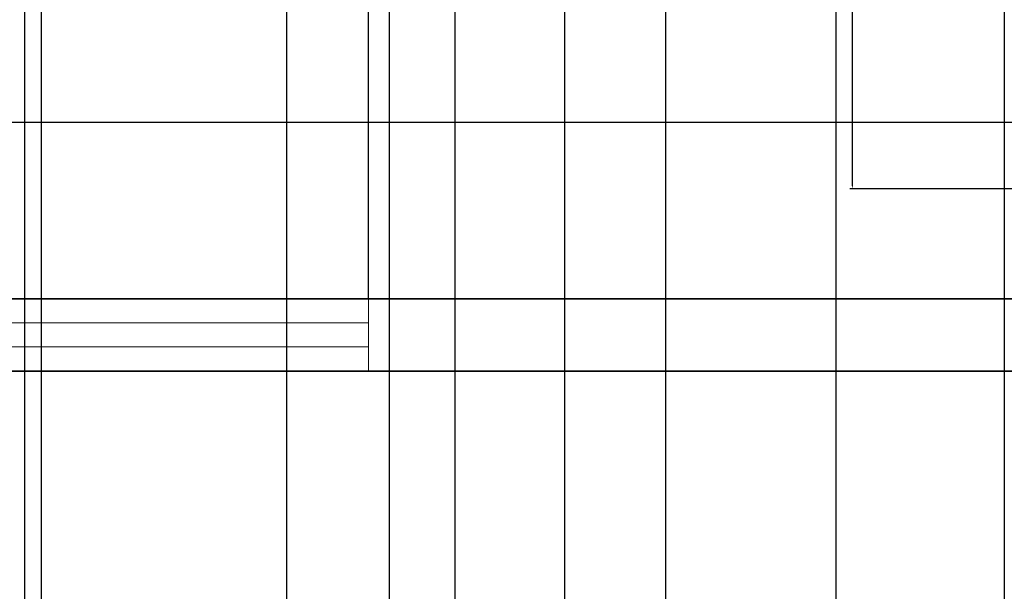
# Model space of a CAD drawing. Units: inches. Extents: x -26 to 385, y 12 to 697.
# Tile 5 of 13: x 223 to 285, y 130 to 165. Entities that reach past the tile are written whole.
import ezdxf

# ---------------------------------------------------------------- set-up
doc = ezdxf.new("R2010")
doc.units = ezdxf.units.IN
doc.header["$MEASUREMENT"] = 0
for name, color, linetype, lineweight in [('A-ANNO-DIMS', 4, 'Continuous', 18), ('A-GLAZ', 5, 'Continuous', 18), ('A-WALL', 40, 'Continuous', 35)]:
    doc.layers.add(name, color=color, linetype=linetype, lineweight=lineweight)
doc.styles.get("Standard").update_dxf_attribs({"font": 'italic8.shx'})
doc.dimstyles.get("Standard").update_dxf_attribs({"dimtxt": 8, "dimasz": 0.18, "dimexe": 0.18, "dimexo": 0.0625, "dimgap": 0.09, "dimtad": 0, "dimtih": 1, "dimtoh": 1, "dimdec": 4, "dimzin": 0, "dimdsep": 46, "dimlunit": 3, "dimtxsty": 'Standard', "dimcen": 0.09, "dimclrd": 2, "dimclre": 3, "dimclrt": 6, "dimadec": 0, "dimazin": 0, "dimtfac": 1, "dimtdec": 4, "dimtofl": 0, "dimtmove": 0, "dimatfit": 3, "dimfxl": 1, "dimtolj": 1, "dimtzin": 0, "dimarcsym": 0})

# ---------------------------------------------------------------- blocks, each defined once
blk = doc.blocks.new('*D11')
at = {"layer": 'A-ANNO-DIMS', "color": 3, "lineweight": -2, "transparency": 16777216}
for p, q in [((285.56, 224.402), (274.992, 224.402)), ((285.56, 154.738), (274.992, 154.738))]:
    blk.add_line(p, q, dxfattribs=at)
at = {"layer": 'A-ANNO-DIMS', "color": 2, "lineweight": -2, "transparency": 16777216}
for p, q in [((275.172, 224.222), (275.172, 195.755)), ((275.172, 154.918), (275.172, 183.384))]:
    blk.add_line(p, q, dxfattribs=at)
at = {"layer": 'A-ANNO-DIMS', "color": 2, "transparency": 16777216}
for points in [[(275.142, 224.222), (275.202, 224.222), (275.172, 224.402)], [(275.142, 154.918), (275.202, 154.918), (275.172, 154.738)]]:
    blk.add_solid(points, dxfattribs=at)
at = {"layer": 'Defpoints', "color": 0, "transparency": 16777216}
for p in [(285.622, 224.402), (275.172, 154.738), (285.622, 154.738)]:
    blk.add_point(p, dxfattribs=at)
at = {"layer": 'A-ANNO-DIMS', "color": 6, "transparency": 16777216, "insert": (275.172, 189.57), "char_height": 8, "attachment_point": 5}
blk.add_mtext('\\A1;SOFA 5\'-9 1/2" TYP.', dxfattribs=at)
blk = doc.blocks.new('*D25')
at = {"layer": 'A-ANNO-DIMS', "color": 3, "lineweight": -2, "transparency": 16777216}
for p, q in [((284.629322, 368.316588), (284.629322, 23.949088)), ((320.629322, 368.316588), (320.629322, 23.949088))]:
    blk.add_line(p, q, dxfattribs=at)
at = {"layer": 'A-ANNO-DIMS', "color": 2, "lineweight": -2, "transparency": 16777216}
for p, q in [((284.449322, 24.129088), (284.269322, 24.129088)), ((320.809322, 24.129088), (320.989322, 24.129088))]:
    blk.add_line(p, q, dxfattribs=at)
at = {"layer": 'A-ANNO-DIMS', "color": 2, "transparency": 16777216}
for points in [[(284.449322, 24.159088), (284.449322, 24.099088), (284.629322, 24.129088)], [(320.809322, 24.159088), (320.809322, 24.099088), (320.629322, 24.129088)]]:
    blk.add_solid(points, dxfattribs=at)
at = {"layer": 'Defpoints', "color": 0, "transparency": 16777216}
for p in [(284.629322, 368.379088), (320.629322, 368.379088), (320.629322, 24.129088)]:
    blk.add_point(p, dxfattribs=at)
at = {"layer": 'A-ANNO-DIMS', "color": 6, "transparency": 16777216, "insert": (302.629322, 24.129088), "char_height": 8, "attachment_point": 5}
blk.add_mtext('\\A1;3\'-0"', dxfattribs=at)
blk = doc.blocks.new('*D28')
at = {"layer": 'A-ANNO-DIMS', "color": 3, "lineweight": -2, "transparency": 16777216}
for p, q in [((141.692, 194.903), (355.559, 194.903)), ((141.692, 158.903), (355.559, 158.903))]:
    blk.add_line(p, q, dxfattribs=at)
at = {"layer": 'A-ANNO-DIMS', "color": 2, "lineweight": -2, "transparency": 16777216}
for p, q in [((355.379, 194.723), (355.379, 181.755)), ((355.379, 159.083), (355.379, 172.052))]:
    blk.add_line(p, q, dxfattribs=at)
at = {"layer": 'A-ANNO-DIMS', "color": 2, "transparency": 16777216}
for points in [[(355.349, 194.723), (355.409, 194.723), (355.379, 194.903)], [(355.349, 159.083), (355.409, 159.083), (355.379, 158.903)]]:
    blk.add_solid(points, dxfattribs=at)
at = {"layer": 'Defpoints', "color": 0, "transparency": 16777216}
for p in [(141.629, 194.903), (355.379, 194.903), (141.629, 158.903)]:
    blk.add_point(p, dxfattribs=at)
at = {"layer": 'A-ANNO-DIMS', "color": 6, "transparency": 16777216, "insert": (355.379, 176.903), "char_height": 8, "attachment_point": 5}
blk.add_mtext('\\A1;3\'-0"', dxfattribs=at)
blk = doc.blocks.new('*D31')
at = {"layer": 'A-ANNO-DIMS', "color": 3, "lineweight": -2, "transparency": 16777216}
for p, q in [((239.888, 166.079), (239.888, 23.949)), ((263.51, 166.079), (263.51, 23.949))]:
    blk.add_line(p, q, dxfattribs=at)
at = {"layer": 'A-ANNO-DIMS', "color": 2, "lineweight": -2, "transparency": 16777216}
for p, q in [((240.068, 24.129), (263.33, 24.129)), ((263.51, 24.129), (263.69, 24.129))]:
    blk.add_line(p, q, dxfattribs=at)
at = {"layer": 'A-ANNO-DIMS', "color": 2, "transparency": 16777216}
for points in [[(240.068, 24.159), (240.068, 24.099), (239.888, 24.129)], [(263.33, 24.159), (263.33, 24.099), (263.51, 24.129)]]:
    blk.add_solid(points, dxfattribs=at)
at = {"layer": 'Defpoints', "color": 0, "transparency": 16777216}
for p in [(239.888, 166.141), (263.51, 166.141), (263.51, 24.129)]:
    blk.add_point(p, dxfattribs=at)
at = {"layer": 'A-ANNO-DIMS', "color": 6, "transparency": 16777216, "insert": (296.732, 24.129), "char_height": 8, "attachment_point": 5}
blk.add_mtext('\\A1;1\'-11 1/2"', dxfattribs=at)
blk = doc.blocks.new('*D35')
at = {"layer": 'A-ANNO-DIMS', "color": 3, "lineweight": -2, "transparency": 16777216}
for p, q in [((193.598, 147.942), (193.598, 684.809)), ((244.986, 147.942), (244.986, 684.809))]:
    blk.add_line(p, q, dxfattribs=at)
at = {"layer": 'A-ANNO-DIMS', "color": 2, "lineweight": -2, "transparency": 16777216}
for p, q in [((193.778, 684.629), (244.806, 684.629)), ((244.986, 684.629), (245.166, 684.629))]:
    blk.add_line(p, q, dxfattribs=at)
at = {"layer": 'A-ANNO-DIMS', "color": 2, "transparency": 16777216}
for points in [[(193.778, 684.659), (193.778, 684.599), (193.598, 684.629)], [(244.806, 684.659), (244.806, 684.599), (244.986, 684.629)]]:
    blk.add_solid(points, dxfattribs=at)
at = {"layer": 'Defpoints', "color": 0, "transparency": 16777216}
for p in [(244.986, 684.629), (193.598, 147.879), (244.986, 147.879)]:
    blk.add_point(p, dxfattribs=at)
at = {"layer": 'A-ANNO-DIMS', "color": 6, "transparency": 16777216, "insert": (278.398, 684.629), "char_height": 8, "attachment_point": 5}
blk.add_mtext('\\A1;4\'-3 1/2"', dxfattribs=at)
blk = doc.blocks.new('*D36')
at = {"layer": 'A-ANNO-DIMS', "color": 3, "lineweight": -2, "transparency": 16777216}
for p, q in [((146.129, 147.942), (146.129, 684.809)), ((193.598, 147.942), (193.598, 684.809))]:
    blk.add_line(p, q, dxfattribs=at)
at = {"layer": 'A-ANNO-DIMS', "color": 2, "lineweight": -2, "transparency": 16777216}
for p, q in [((146.309, 684.629), (193.418, 684.629)), ((193.598, 684.629), (193.778, 684.629))]:
    blk.add_line(p, q, dxfattribs=at)
at = {"layer": 'A-ANNO-DIMS', "color": 2, "transparency": 16777216}
for points in [[(146.309, 684.659), (146.309, 684.599), (146.129, 684.629)], [(193.418, 684.659), (193.418, 684.599), (193.598, 684.629)]]:
    blk.add_solid(points, dxfattribs=at)
at = {"layer": 'Defpoints', "color": 0, "transparency": 16777216}
for p in [(193.598, 684.629), (146.129, 147.879), (193.598, 147.879)]:
    blk.add_point(p, dxfattribs=at)
at = {"layer": 'A-ANNO-DIMS', "color": 6, "transparency": 16777216, "insert": (228.344, 684.629), "char_height": 8, "attachment_point": 5}
blk.add_mtext('\\A1;3\'-11 1/2"', dxfattribs=at)
blk = doc.blocks.new('*D37')
at = {"layer": 'A-ANNO-DIMS', "color": 3, "lineweight": -2, "transparency": 16777216}
for p, q in [((223.549, 597.317), (223.549, 23.949)), ((257.22, 597.317), (257.22, 23.949))]:
    blk.add_line(p, q, dxfattribs=at)
at = {"layer": 'A-ANNO-DIMS', "color": 2, "lineweight": -2, "transparency": 16777216}
for p, q in [((223.729, 24.129), (257.04, 24.129)), ((257.22, 24.129), (257.4, 24.129))]:
    blk.add_line(p, q, dxfattribs=at)
at = {"layer": 'A-ANNO-DIMS', "color": 2, "transparency": 16777216}
for points in [[(223.729, 24.159), (223.729, 24.099), (223.549, 24.129)], [(257.04, 24.159), (257.04, 24.099), (257.22, 24.129)]]:
    blk.add_solid(points, dxfattribs=at)
at = {"layer": 'Defpoints', "color": 0, "transparency": 16777216}
for p in [(223.549, 597.379), (257.22, 597.379), (257.22, 24.129)]:
    blk.add_point(p, dxfattribs=at)
at = {"layer": 'A-ANNO-DIMS', "color": 6, "transparency": 16777216, "insert": (290.633, 24.129), "char_height": 8, "attachment_point": 5}
blk.add_mtext('\\A1;2\'-9 1/2"', dxfattribs=at)
blk = doc.blocks.new('*D39')
at = {"layer": 'A-ANNO-DIMS', "color": 3, "lineweight": -2, "transparency": 16777216}
for p, q in [((183.359, 597.317), (183.359, 23.949)), ((213.359, 597.317), (213.359, 23.949))]:
    blk.add_line(p, q, dxfattribs=at)
at = {"layer": 'A-ANNO-DIMS', "color": 2, "lineweight": -2, "transparency": 16777216}
for p, q in [((183.539, 24.129), (213.179, 24.129)), ((213.359, 24.129), (213.539, 24.129))]:
    blk.add_line(p, q, dxfattribs=at)
at = {"layer": 'A-ANNO-DIMS', "color": 2, "transparency": 16777216}
for points in [[(183.539, 24.159), (183.539, 24.099), (183.359, 24.129)], [(213.179, 24.159), (213.179, 24.099), (213.359, 24.129)]]:
    blk.add_solid(points, dxfattribs=at)
at = {"layer": 'Defpoints', "color": 0, "transparency": 16777216}
for p in [(183.359, 597.379), (213.359, 597.379), (213.359, 24.129)]:
    blk.add_point(p, dxfattribs=at)
at = {"layer": 'A-ANNO-DIMS', "color": 6, "transparency": 16777216, "insert": (231.533, 24.129), "char_height": 8, "attachment_point": 5}
blk.add_mtext('\\A1;2\'-6"', dxfattribs=at)
blk = doc.blocks.new('*D42')
at = {"layer": 'A-ANNO-DIMS', "color": 3, "lineweight": -2, "transparency": 16777216}
for p, q in [((250.371, 518.992), (250.371, 23.949)), ((274.129, 518.992), (274.129, 23.949))]:
    blk.add_line(p, q, dxfattribs=at)
at = {"layer": 'A-ANNO-DIMS', "color": 2, "lineweight": -2, "transparency": 16777216}
for p, q in [((250.551, 24.129), (273.949, 24.129)), ((274.129, 24.129), (274.309, 24.129))]:
    blk.add_line(p, q, dxfattribs=at)
at = {"layer": 'A-ANNO-DIMS', "color": 2, "transparency": 16777216}
for points in [[(250.551, 24.159), (250.551, 24.099), (250.371, 24.129)], [(273.949, 24.159), (273.949, 24.099), (274.129, 24.129)]]:
    blk.add_solid(points, dxfattribs=at)
at = {"layer": 'Defpoints', "color": 0, "transparency": 16777216}
for p in [(250.371, 519.055), (274.129, 519.055), (274.129, 24.129)]:
    blk.add_point(p, dxfattribs=at)
at = {"layer": 'A-ANNO-DIMS', "color": 6, "transparency": 16777216, "insert": (292.304, 24.129), "char_height": 8, "attachment_point": 5}
blk.add_mtext('\\A1;2\'-0"', dxfattribs=at)
blk = doc.blocks.new('*D46')
at = {"layer": 'A-ANNO-DIMS', "color": 3, "lineweight": -2, "transparency": 16777216}
for p, q in [((224.595, 477.317), (224.595, 23.949)), ((284.629, 477.317), (284.629, 23.949))]:
    blk.add_line(p, q, dxfattribs=at)
at = {"layer": 'A-ANNO-DIMS', "color": 2, "lineweight": -2, "transparency": 16777216}
for p, q in [((224.775, 24.129), (236.617, 24.129)), ((284.449, 24.129), (272.607, 24.129))]:
    blk.add_line(p, q, dxfattribs=at)
at = {"layer": 'A-ANNO-DIMS', "color": 2, "transparency": 16777216}
for points in [[(224.775, 24.159), (224.775, 24.099), (224.595, 24.129)], [(284.449, 24.159), (284.449, 24.099), (284.629, 24.129)]]:
    blk.add_solid(points, dxfattribs=at)
at = {"layer": 'Defpoints', "color": 0, "transparency": 16777216}
for p in [(224.595, 477.379), (284.629, 477.379), (284.629, 24.129)]:
    blk.add_point(p, dxfattribs=at)
at = {"layer": 'A-ANNO-DIMS', "color": 6, "transparency": 16777216, "insert": (254.612, 24.129), "char_height": 8, "attachment_point": 5}
blk.add_mtext('\\A1;5\'-0"', dxfattribs=at)
blk = doc.blocks.new('*D50')
at = {"layer": 'A-ANNO-DIMS', "color": 3, "lineweight": -2, "transparency": 16777216}
for p, q in [((246.278, 401.871), (246.278, 23.949)), ((284.629, 398.317), (284.629, 23.949))]:
    blk.add_line(p, q, dxfattribs=at)
at = {"layer": 'A-ANNO-DIMS', "color": 2, "lineweight": -2, "transparency": 16777216}
for p, q in [((246.458, 24.129), (284.449, 24.129)), ((284.629, 24.129), (284.809, 24.129))]:
    blk.add_line(p, q, dxfattribs=at)
at = {"layer": 'A-ANNO-DIMS', "color": 2, "transparency": 16777216}
for points in [[(246.458, 24.159), (246.458, 24.099), (246.278, 24.129)], [(284.449, 24.159), (284.449, 24.099), (284.629, 24.129)]]:
    blk.add_solid(points, dxfattribs=at)
at = {"layer": 'Defpoints', "color": 0, "transparency": 16777216}
for p in [(246.278, 401.934), (284.629, 398.379), (284.629, 24.129)]:
    blk.add_point(p, dxfattribs=at)
at = {"layer": 'A-ANNO-DIMS', "color": 6, "transparency": 16777216, "insert": (318.042, 24.129), "char_height": 8, "attachment_point": 5}
blk.add_mtext('\\A1;3\'-2 1/2"', dxfattribs=at)
blk = doc.blocks.new('*D55')
at = {"layer": 'A-ANNO-DIMS', "color": 3, "lineweight": -2, "transparency": 16777216}
for p, q in [((146.192, 158.903), (355.559, 158.903)), ((146.192, 147.879), (355.559, 147.879))]:
    blk.add_line(p, q, dxfattribs=at)
at = {"layer": 'A-ANNO-DIMS', "color": 2, "lineweight": -2, "transparency": 16777216}
for p, q in [((355.379, 158.723), (355.379, 158.243)), ((355.379, 148.059), (355.379, 148.539))]:
    blk.add_line(p, q, dxfattribs=at)
at = {"layer": 'A-ANNO-DIMS', "color": 2, "transparency": 16777216}
for points in [[(355.349, 158.723), (355.409, 158.723), (355.379, 158.903)], [(355.349, 148.059), (355.409, 148.059), (355.379, 147.879)]]:
    blk.add_solid(points, dxfattribs=at)
at = {"layer": 'Defpoints', "color": 0, "transparency": 16777216}
for p in [(146.129, 158.903), (355.379, 158.903), (146.129, 147.879)]:
    blk.add_point(p, dxfattribs=at)
at = {"layer": 'A-ANNO-DIMS', "color": 6, "transparency": 16777216, "insert": (355.379, 153.391), "char_height": 8, "attachment_point": 5}
blk.add_mtext('\\A1;0\'-11"', dxfattribs=at)

msp = doc.modelspace()

# ---------------------------------------------------------------- linework, layer by layer
at = {"layer": 'A-GLAZ'}
for p, q in [((244.98557, 147.87909), (193.59818, 147.87909)), ((244.98557, 143.37909), (244.98557, 147.87909)), ((193.59818, 146.37909), (244.98557, 146.37909)), ((193.59818, 144.87909), (244.98557, 144.87909)), ((193.59818, 143.37909), (244.98557, 143.37909))]:
    msp.add_line(p, q, dxfattribs=at)
at = {"layer": 'A-WALL'}
for p, q in [((320.62932, 147.87909), (146.12932, 147.87909)), ((320.62932, 143.37909), (141.62932, 143.37909))]:
    msp.add_line(p, q, dxfattribs=at)

# ---------------------------------------------------------------- dimensions: what is measured, and where the dimension line sits
at = {"layer": 'A-ANNO-DIMS'}
for base, p1, p2, picture, middle in [((193.59818, 684.62909), (146.12932, 147.87909), (193.59818, 147.87909), '*D36', (228.34437, 684.62909)), ((244.98557, 684.62909), (193.59818, 147.87909), (244.98557, 147.87909), '*D35', (278.39843, 684.62909)), ((213.35855, 24.12909), (183.35855, 597.37909), (213.35855, 597.37909), '*D39', (231.53331, 24.12909)), ((257.21981, 24.12909), (223.54856, 597.37909), (257.21981, 597.37909), '*D37', (290.63267, 24.12909)), ((274.12932, 24.12909), (250.37102, 519.05498), (274.12932, 519.05498), '*D42', (292.30408, 24.12909)), ((284.62932, 24.12909), (224.59493, 477.37909), (284.62932, 477.37909), '*D46', (254.61213, 24.12909)), ((284.62932, 24.12909), (246.27828, 401.934), (284.62932, 398.37909), '*D50', (318.04218, 24.12909)), ((320.62932, 24.12909), (284.62932, 368.37909), (320.62932, 368.37909), '*D25', (302.62932, 24.12909)), ((263.50956, 24.12909), (239.88756, 166.14113), (263.50956, 166.14113), '*D31', (296.73194, 24.12909))]:
    dim = msp.add_linear_dim(base=base, p1=p1, p2=p2, dimstyle='Standard', override={"dimdec": 1, "dimlfac": 1, "dimrnd": 0, "dimzin": 1, "dimdsep": 46, "dimlunit": 4, "dimfrac": 2}, dxfattribs=at)
    dim.commit()
    dim.dimension.update_dxf_attribs({"geometry": picture, "text_midpoint": middle})
dim = msp.add_linear_dim(base=(275.17245, 154.73754), p1=(285.62207, 224.40165), p2=(285.62207, 154.73754), angle=270, text='SOFA <> TYP.', dimstyle='Standard', override={"dimdec": 1, "dimlfac": 1, "dimrnd": 0, "dimzin": 1, "dimdsep": 46, "dimlunit": 4, "dimfrac": 2}, dxfattribs=at)
dim.commit()
dim.dimension.update_dxf_attribs({"geometry": '*D11', "text_midpoint": (275.17245, 189.56959)})
for base, p1, p2, picture, middle in [((355.37932, 194.90341), (141.62932, 158.90341), (141.62932, 194.90341), '*D28', (355.37932, 176.90341)), ((355.37932, 158.90341), (146.12932, 147.87909), (146.12932, 158.90341), '*D55', (355.37932, 153.39125))]:
    dim = msp.add_linear_dim(base=base, p1=p1, p2=p2, angle=90, dimstyle='Standard', override={"dimdec": 1, "dimlfac": 1, "dimrnd": 0, "dimzin": 1, "dimdsep": 46, "dimlunit": 4, "dimfrac": 2}, dxfattribs=at)
    dim.commit()
    dim.dimension.update_dxf_attribs({"geometry": picture, "text_midpoint": middle})

doc.saveas('drawing.dxf')
